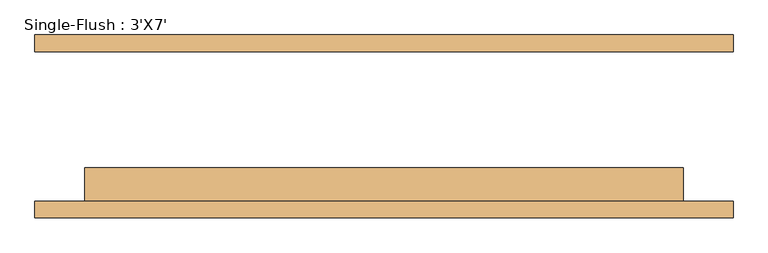
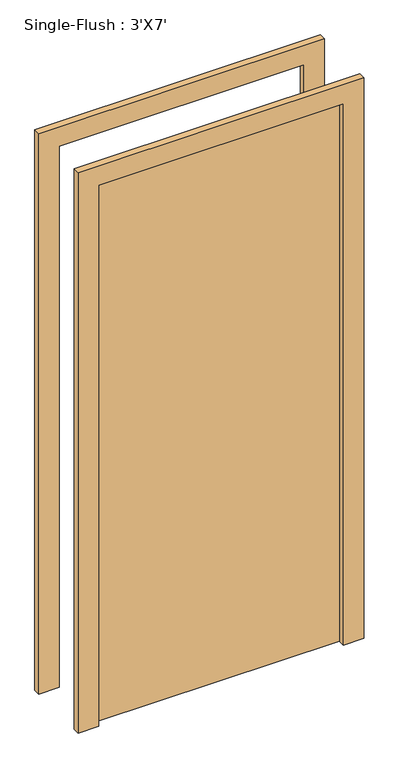
"""IFC4 building model written with IfcOpenShell, lengths in millimetres: door geometry, Single-Flush : 3'X7'."""

from ifc_helpers import new_model, si_unit, frame, origin, origin_with_axes, place, context, project, spatial, polyline, outline, extrude, source, transform, mapped, element, save


def single_flush_3_x7_a90ba1ad(model_context):
    return source(origin(), model_context, "Body", "SweptSolid", [
        extrude(outline(polyline([(2209.8, -533.4), (0.0, -533.4), (0.0, -457.2), (2133.6, -457.2), (2133.6, 457.2), (0.0, 457.2), (0.0, 533.4), (2209.8, 533.4), (2209.8, -533.4)])), frame((0.0, -139.7, 0.0), z_axis=(0.0, 1.0, 0.0), x_axis=(0.0, 0.0, 1.0)), (0.0, 0.0, 1.0), 25.4),
        extrude(outline(polyline([(2209.8, 533.4), (2209.8, -533.4), (0.0, -533.4), (0.0, -457.2), (2133.6, -457.2), (2133.6, 457.2), (0.0, 457.2), (0.0, 533.4), (2209.8, 533.4)])), frame((0.0, 114.3, 0.0), z_axis=(0.0, 1.0, 0.0), x_axis=(0.0, 0.0, 1.0)), (0.0, 0.0, 1.0), 25.4),
        extrude(outline(polyline([(457.2, -63.5), (457.2, -114.3), (-457.2, -114.3), (-457.2, -63.5), (457.2, -63.5)])), origin_with_axes(), (0.0, 0.0, 1.0), 2133.6),
    ])


if __name__ == "__main__":
    model = new_model("IFC4")
    model_context = context("Model", 3, world=origin())
    ifc_project = project(units=[si_unit("LENGTHUNIT", "METRE", prefix="MILLI")], contexts=[model_context])
    site = spatial("IfcSite", under=ifc_project)
    building = spatial("IfcBuilding", under=site)
    placement = place(None, origin())
    single_flush_3_x7_shape = single_flush_3_x7_a90ba1ad(model_context)
    element("IfcDoor", 1, ObjectType="Single-Flush : 3'X7'", at=placement, inside=building, context=model_context, shape_type="MappedRepresentation", body=[
        mapped(single_flush_3_x7_shape, transform((0.0, 0.0, 0.0), x_axis=(1.0, 0.0, 0.0), y_axis=(0.0, 1.0, 0.0), z_axis=(0.0, 0.0, 1.0))),
    ])
    save(model, "model.ifc")

# Revit data of these elements
# Type "Single-Flush : 3'X7'"
#   Type Mark = "8"
#   Construction Type Id = "MDOOR"
#   Assembly Code = "C1020"
#   Analytic Construction = "Metal"
#   Thickness = 0' - 2"
#   Heat Transfer Coefficient (U) = 0.651978 BTU/(h·ft²·°F)
#   Height = 7' - 0"
#   Trim Projection Ext = 0' - 1"
#   Trim Projection Int = 0' - 1"
#   Trim Width = 0' - 3"
#   Width = 3' - 0"
#   Define Thermal Properties by = 1
#   Door Material = Door - Panel
#   Frame Material = Door - Frame
#   Visual Light Transmittance = 0
#   Solar Heat Gain Coefficient = 0
#   Function = (empty or 0)
#   Wall Closure = (empty or 0)
# Element 1 (IfcDoor, "Single-Flush : 3'X7'")
#   Materials on its faces: "Door - Frame", "Door - Panel"
# Materials
#   "Door - Panel": class "Wood", colour RGB 210 159 95, transparency 0, Cost = 0
#   "Door - Frame": colour RGB 118 70 51, transparency 0, Cost = 0
